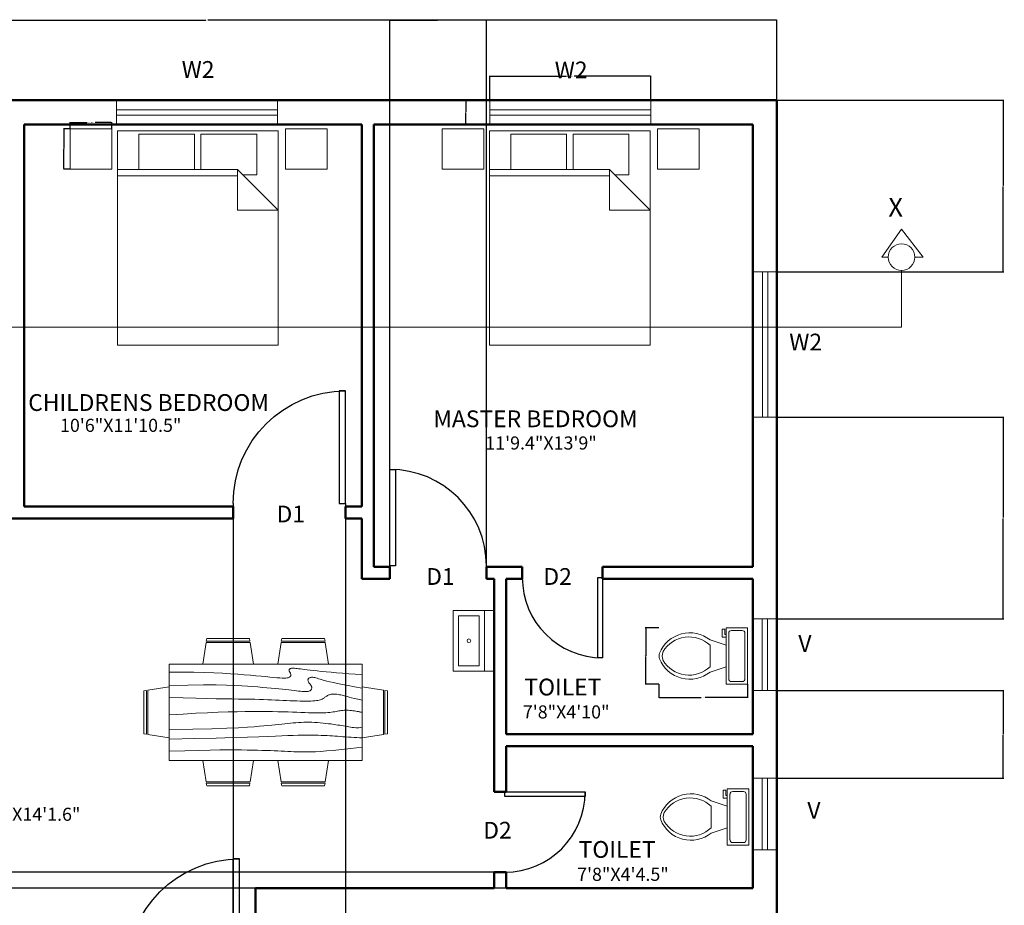
# Model space of a CAD drawing. Units: inches. Extents: x 7359 to 7979, y 33027 to 34263.
# Tile 32 of 32: x 7601 to 7969, y 33933 to 34263. Entities that reach past the tile are written whole.
import ezdxf

# ---------------------------------------------------------------- set-up
doc = ezdxf.new("R2010")
doc.units = ezdxf.units.IN
for name, color, linetype, lineweight in [('A-ANNO-DIMS', 2, 'Continuous', 18), ('A-ANNO-SYMB', 7, 'Continuous', 18), ('A-ANNO-TEXT', 3, 'Continuous', 18), ('A-AREA-IDEN', 7, 'Continuous', 18), ('A-DOOR', 3, 'Continuous', 25), ('A-FLOR-FIXT', 9, 'Continuous', 18), ('A-FURN', 8, 'Continuous', 18), ('A-GLAZ', 4, 'Continuous', 18), ('A-WALL', 7, 'Continuous', 50)]:
    doc.layers.add(name, color=color, linetype=linetype, lineweight=lineweight)
doc.styles.get("Standard").update_dxf_attribs({"font": 'arial.ttf'})
doc.dimstyles.get("Standard").update_dxf_attribs({"dimtxt": 0.18, "dimasz": 0.18, "dimexe": 0.18, "dimexo": 0.0625, "dimgap": 0.09, "dimtad": 0, "dimtih": 1, "dimtoh": 1, "dimdec": 4, "dimzin": 0, "dimdsep": 46, "dimtxsty": 'Standard', "dimcen": 0.09, "dimadec": 0, "dimazin": 0, "dimtfac": 1, "dimtdec": 4, "dimtofl": 0, "dimtmove": 0, "dimatfit": 3, "dimfxl": 1, "dimtolj": 1, "dimtzin": 0, "dimarcsym": 0})

# ---------------------------------------------------------------- blocks, each defined once
blk = doc.blocks.new('*U2')
for p, q in [((0, 0), (0, -100)), ((750, 0), (750, -100))]:
    blk.add_line(p, q)
blk.add_lwpolyline([(0, 0), (0, 750), (43.75, 750), (43.75, 0)], close=True)
blk.add_arc((0, 0), 750, 0, 90)
blk = doc.blocks.new('Dining Set - 36 x 72 in.')
for p, q in [((-22.2343, 26.00059), (-23.4847, 17.99762)), ((-22.2304, 26), (-5.7608, 26)), ((-22, 27.5), (-22.1562, 26.50042)), ((-5.8416, 26.5), (-22.1534, 26.5)), ((-22, 27.5), (-6, 27.5)), ((-5.8437, 26.49966), (-6, 27.5)), ((-4.5152, 17.99762), (-5.7655, 25.99926)), ((5.7657, 26.00059), (4.5153, 17.99762)), ((5.7696, 26), (22.2392, 26)), ((6, 27.5), (5.8438, 26.50042)), ((22.1584, 26.5), (5.8466, 26.5)), ((6, 27.5), (22, 27.5)), ((22.1563, 26.49966), (22, 27.5)), ((23.4848, 17.99762), (22.2345, 25.99926)), ((36, 18), (-36, 18)), ((-36, 18), (-36, -18)), ((36, -18), (36, 18)), ((-45.5, 8), (-44.5004, 8.15617)), ((-45.5, 8), (-45.5, -8)), ((-44.5, -8.15843), (-44.5, 8.15338)), ((-44.0006, 8.23428), (-35.9976, 9.48474)), ((-44, 8.23041), (-44, -8.23915)), ((44.0006, 8.23428), (35.9976, 9.48474)), ((44, 8.23041), (44, -8.23915)), ((44.5, -8.15843), (44.5, 8.15338)), ((45.5, 8), (44.5005, 8.15617)), ((45.5, 8), (45.5, -8)), ((-44.4997, -8.15631), (-45.5, -8)), ((-35.9976, -9.48476), (-43.9993, -8.2345)), ((35.9976, -9.48476), (43.9993, -8.2345)), ((44.4997, -8.15631), (45.5, -8)), ((-36, -18), (36, -18)), ((-22.2343, -26.0006), (-23.4847, -17.99762)), ((-4.5152, -17.99762), (-5.7655, -25.99928)), ((5.7657, -26.0006), (4.5153, -17.99762)), ((23.4848, -17.99762), (22.2345, -25.99928)), ((-22.2304, -26), (-5.7608, -26)), ((-22, -27.5), (-22.1562, -26.50044)), ((-5.8416, -26.5), (-22.1534, -26.5)), ((-22, -27.5), (-6, -27.5)), ((-5.8437, -26.49967), (-6, -27.5)), ((5.7696, -26), (22.2392, -26)), ((6, -27.5), (5.8438, -26.50044)), ((22.1584, -26.5), (5.8466, -26.5)), ((6, -27.5), (22, -27.5)), ((22.1563, -26.49967), (22, -27.5))]:
    blk.add_line(p, q)
for points in [[(-36, 15), (-31.1772, 14.97754), (-26.8079, 14.91406), (-22.8538, 14.81543), (-19.276, 14.6875), (-16.0362, 14.53613), (-13.0957, 14.36718), (-10.4159, 14.18652), (-7.9583, 14), (-5.6904, 13.81315), (-3.6035, 13.63021), (-1.6954, 13.45508), (0.0365, 13.29166), (1.5945, 13.14388), (2.9811, 13.01562), (4.1988, 12.9108), (5.25, 12.83333), (6.1393, 12.78613), (6.8802, 12.76823), (7.4883, 12.77767), (7.9792, 12.8125), (8.3685, 12.87077), (8.6719, 12.95052), (8.9049, 13.0498), (9.0833, 13.16666), (9.2205, 13.29899), (9.3216, 13.44401), (9.3895, 13.59879), (9.4271, 13.76041), (9.4373, 13.92594), (9.4232, 14.09245), (9.3875, 14.257), (9.3333, 14.41666), (9.2638, 14.56917), (9.1836, 14.71484), (9.0975, 14.85465), (9.0104, 14.98958), (8.9272, 15.1206), (8.8529, 15.2487), (8.7922, 15.37483), (8.75, 15.5), (8.7305, 15.62467), (8.7344, 15.74739), (8.7617, 15.86621), (8.8125, 15.97916), (8.8867, 16.08431), (8.9844, 16.17968), (9.1055, 16.26334), (9.25, 16.33333), (9.4189, 16.38802), (9.6172, 16.42708), (9.8506, 16.45052), (10.125, 16.45833), (10.4463, 16.45052), (10.8203, 16.42708), (11.2529, 16.38802), (11.75, 16.33333), (12.3184, 16.26318), (12.9694, 16.17838), (13.7151, 16.07991), (14.5677, 15.96875), (15.5395, 15.84586), (16.6426, 15.71224), (17.8893, 15.56884), (19.2917, 15.41666), (20.859, 15.25667), (22.5879, 15.08984), (24.4721, 14.91715), (26.5052, 14.73958), (28.6809, 14.5581), (30.9929, 14.3737), (33.4347, 14.18733), (36, 14)], [(-36, 10), (-28.9766, 10.14274), (-23.1725, 10.20442), (-18.4241, 10.19775), (-14.5677, 10.13541), (-11.4399, 10.03011), (-8.877, 9.89453), (-6.7154, 9.74137), (-4.7917, 9.58333), (-2.9698, 9.43082), (-1.2246, 9.28515), (0.4415, 9.14534), (2.026, 9.01041), (3.5266, 8.87939), (4.9408, 8.7513), (6.266, 8.62516), (7.5, 8.5), (8.6411, 8.37549), (9.6914, 8.2539), (10.6538, 8.13818), (11.5312, 8.03125), (12.3267, 7.93603), (13.043, 7.85547), (13.6831, 7.79248), (14.25, 7.75), (14.7471, 7.7303), (15.1797, 7.73307), (15.5537, 7.75732), (15.875, 7.80208), (16.1494, 7.86637), (16.3828, 7.94922), (16.5811, 8.04964), (16.75, 8.16666), (16.8944, 8.29915), (17.0143, 8.44531), (17.1089, 8.60319), (17.1771, 8.77083), (17.218, 8.94629), (17.2305, 9.1276), (17.2137, 9.31282), (17.1667, 9.5), (17.0895, 9.6875), (16.987, 9.875), (16.8649, 10.0625), (16.7292, 10.25), (16.5856, 10.4375), (16.4401, 10.625), (16.2985, 10.8125), (16.1667, 11), (16.05, 11.18733), (15.9518, 11.3737), (15.8752, 11.5581), (15.8229, 11.73958), (15.798, 11.91715), (15.8034, 12.08984), (15.842, 12.25667), (15.9167, 12.41666), (16.0295, 12.56836), (16.1784, 12.70833), (16.3605, 12.83268), (16.5729, 12.9375), (16.8127, 13.01888), (17.0768, 13.07291), (17.3625, 13.0957), (17.6667, 13.08333), (17.9894, 13.03312), (18.3418, 12.94726), (18.7382, 12.82918), (19.1927, 12.68229), (19.7195, 12.51001), (20.3327, 12.31575), (21.0465, 12.10294), (21.875, 11.875), (22.8357, 11.63354), (23.959, 11.37304), (25.2786, 11.08618), (26.8282, 10.76562), (28.6414, 10.40405), (30.752, 9.99414), (33.1936, 9.52856), (36, 9)], [(-36, 5.5), (-30.7157, 5.3348), (-26.069, 5.20963), (-21.9946, 5.11767), (-18.4271, 5.05208), (-15.3009, 5.00602), (-12.5508, 4.97265), (-10.1112, 4.94515), (-7.9167, 4.91666), (-5.909, 4.88167), (-4.0586, 4.83984), (-2.3429, 4.79215), (-0.7396, 4.73958), (0.7739, 4.6831), (2.22, 4.6237), (3.6213, 4.56233), (5, 4.5), (6.373, 4.43782), (7.7344, 4.3776), (9.0723, 4.32129), (10.375, 4.27083), (11.6309, 4.22819), (12.8281, 4.19531), (13.9551, 4.17415), (15, 4.16666), (15.954, 4.17448), (16.819, 4.19791), (17.6001, 4.23698), (18.3021, 4.29166), (18.9299, 4.36198), (19.4883, 4.44791), (19.9823, 4.54948), (20.4167, 4.66666), (20.7969, 4.79899), (21.1302, 4.94401), (21.4245, 5.09879), (21.6875, 5.26041), (21.9271, 5.42594), (22.1511, 5.59245), (22.3672, 5.757), (22.5834, 5.91666), (22.8065, 6.06868), (23.0404, 6.21093), (23.2879, 6.34147), (23.5521, 6.45833), (23.8358, 6.55957), (24.142, 6.64323), (24.4735, 6.70735), (24.8334, 6.75), (25.2235, 6.76969), (25.642, 6.76692), (26.0858, 6.74267), (26.5521, 6.69791), (27.0379, 6.63362), (27.5404, 6.55078), (28.0565, 6.45036), (28.5834, 6.33333), (29.1242, 6.19987), (29.7071, 6.04687), (30.3661, 5.87044), (31.1354, 5.66666), (32.0493, 5.43164), (33.142, 5.16146), (34.4475, 4.85221), (36, 4.5)], [(-36, -1), (-30.7915, -0.6591), (-26.0195, -0.38216), (-21.6519, -0.16284), (-17.6563, 0.00521), (-14.0005, 0.12833), (-10.6523, 0.21289), (-7.5796, 0.26522), (-4.75, 0.29166), (-2.134, 0.29793), (0.2878, 0.28711), (2.5317, 0.26163), (4.6146, 0.22396), (6.5529, 0.17651), (8.3633, 0.12174), (10.0623, 0.06209), (11.6667, 0), (13.1899, -0.06201), (14.6341, -0.1211), (15.9982, -0.17432), (17.2813, -0.21875), (18.4823, -0.25147), (19.6003, -0.26953), (20.6343, -0.27002), (21.5834, -0.25), (22.4481, -0.20768), (23.2357, -0.14584), (23.9549, -0.06836), (24.6146, 0.02083), (25.2235, 0.11784), (25.7904, 0.21875), (26.3241, 0.31966), (26.8334, 0.41666), (27.3265, 0.50618), (27.8099, 0.58593), (28.2894, 0.65397), (28.7709, 0.70833), (29.2601, 0.74707), (29.763, 0.76823), (30.2855, 0.76985), (30.8334, 0.75), (31.4088, 0.70784), (31.9994, 0.64713), (32.589, 0.57275), (33.1615, 0.48958), (33.7008, 0.4025), (34.1908, 0.3164), (34.6153, 0.23616), (34.9584, 0.16666), (35.2099, 0.11165), (35.3848, 0.07031), (35.504, 0.04069), (35.5886, 0.02083), (35.6594, 0.00879), (35.7377, 0.0026), (35.8442, 0.00032), (36, 0)], [(-36, -6.5), (-27.1843, -6.31267), (-20.084, -6.1263), (-14.469, -5.9419), (-10.1094, -5.76042), (-6.7752, -5.58285), (-4.2363, -5.41016), (-2.2629, -5.24333), (-0.625, -5.08334), (0.8708, -4.93099), (2.2715, -4.78646), (3.5872, -4.64974), (4.8281, -4.52084), (6.0046, -4.39974), (7.127, -4.28646), (8.2053, -4.18099), (9.25, -4.08334), (10.2705, -3.99382), (11.2734, -3.91407), (12.2647, -3.84603), (13.25, -3.79167), (14.2354, -3.75293), (15.2266, -3.73177), (16.2295, -3.73015), (17.25, -3.75), (18.2912, -3.79248), (19.3451, -3.85547), (20.4009, -3.93604), (21.4479, -4.03125), (22.4754, -4.13819), (23.4727, -4.25391), (24.4289, -4.37549), (25.3334, -4.5), (26.1785, -4.62492), (26.9694, -4.74935), (27.7145, -4.87281), (28.4219, -4.99479), (29.1, -5.11483), (29.7572, -5.23242), (30.4016, -5.34709), (31.0417, -5.45834), (31.6837, -5.56437), (32.3262, -5.65821), (32.9658, -5.73153), (33.599, -5.77604), (34.2224, -5.78345), (34.8327, -5.74545), (35.4264, -5.65373), (36, -5.5)], [(-36, -10), (-26.4022, -9.81299), (-18.4675, -9.62891), (-11.9839, -9.45069), (-6.7396, -9.28125), (-2.5226, -9.12354), (0.8789, -8.98047), (3.6769, -8.85498), (6.0833, -8.75), (8.2767, -8.66765), (10.3021, -8.60677), (12.1712, -8.56543), (13.8958, -8.54167), (15.4876, -8.53353), (16.9583, -8.53907), (18.3197, -8.55632), (19.5834, -8.58334), (20.7616, -8.61841), (21.8685, -8.66081), (22.9188, -8.71004), (23.9271, -8.76563), (24.9081, -8.82707), (25.8763, -8.89388), (26.8465, -8.96558), (27.8334, -9.04167), (28.8474, -9.12118), (29.8828, -9.20117), (30.93, -9.27824), (31.9792, -9.34896), (33.0205, -9.40991), (34.0443, -9.45768), (35.0407, -9.48885), (36, -9.5)], [(-36, -14.5), (-30.0881, -14.33513), (-25.0332, -14.21224), (-20.7312, -14.12647), (-17.0781, -14.07292), (-13.97, -14.04671), (-11.3027, -14.04297), (-8.9724, -14.05681), (-6.875, -14.08334), (-4.9224, -14.11833), (-3.0905, -14.16016), (-1.3709, -14.20785), (0.2448, -14.26042), (1.7647, -14.3169), (3.1973, -14.3763), (4.5507, -14.43767), (5.8333, -14.5), (7.0554, -14.5621), (8.235, -14.62175), (9.3922, -14.67652), (10.5469, -14.72396), (11.7192, -14.76164), (12.929, -14.78711), (14.1965, -14.79794), (15.5417, -14.79167), (16.9933, -14.76424), (18.6152, -14.70508), (20.4804, -14.60197), (22.6615, -14.44271), (25.2312, -14.21509), (28.2624, -13.9069), (31.8277, -13.50594), (36, -13)]]:
    blk.add_lwpolyline(points)
blk = doc.blocks.new('Bed - Queen')
for p, q in [((0, -80.00003), (0, 0)), ((0, 0), (59.99999, 0)), ((59.99999, 0), (59.99999, -80.00003)), ((7.99999, -1.2), (28.79998, -1.2)), ((7.99999, -14.4), (7.99999, -1.2)), ((28.79998, -1.2), (28.79998, -14.4)), ((31.19999, -1.2), (51.99999, -1.2)), ((31.19999, -14.4), (31.19999, -1.2)), ((51.99999, -1.2), (51.99999, -16.4)), ((0, -14.4), (44.8, -14.4)), ((59.99999, -29.6), (44.8, -14.4)), ((44.8, -14.4), (44.8, -29.6)), ((44.8, -16.8), (0, -16.8)), ((51.99999, -16.4), (46.79936, -16.4)), ((44.8, -29.6), (59.99999, -29.6)), ((59.99999, -80.00003), (0, -80.00003))]:
    blk.add_line(p, q)
blk = doc.blocks.new('Toilet - top')
for p, q in [((9.5, -6), (9.5, -2)), ((-10, -8.5), (-8, -8.5)), ((-10, -9.5), (-10, -8.5)), ((-7, -9.5), (-10, -9.5)), ((-8, -8.5), (-8, -8)), ((-7, -8), (-7, -9.5)), ((-4, -8), (-6, -14)), ((4, -8), (6, -14)), ((4, -14), (-4, -14))]:
    blk.add_line(p, q)
blk.add_lwpolyline([(10.5, -8), (10.5, 0), (-10.5, 0), (-10.5, -8)], close=True)
for points in [[(-9.5, -2), (-9.5, -6)], [(8.5, -1), (-8.5, -1)], [(-8.5, -7), (8.5, -7)]]:
    blk.add_lwpolyline(points)
for centre, radius, start, end in [((-8.62, -1.88), 0.884, 81.8699, 188.1301), ((8.62, -1.88), 0.884, 351.8699, 98.1301), ((-8.62, -6.12), 0.884, 171.8699, 278.1301), ((8.62, -6.12), 0.884, 261.8699, 8.1301), ((3.52, -21.58), 12.17, 141.4691, 247.9714), ((4.2, -21.82), 11.33, 136.3677, 238.9468), ((-3.52, -21.58), 12.17, 292.0284, 38.5307), ((-4.2, -21.82), 11.33, 301.053, 43.6321), ((0, -27.88), 4, 245.7318, 294.2682), ((0, -29), 4, 254.8605, 285.1395)]:
    blk.add_arc(centre, radius, start, end)
blk = doc.blocks.new('TABLE-BEDSIDE')
blk.add_lwpolyline([(0, 15), (15.54, 15), (15.54, 0), (0, 0)], close=True)
blk = doc.blocks.new('BASIN-WALL')
for points in [[(11.75, 22.71), (0, 22.71), (0, 0), (11.75, 0)], [(15.29, 22.71), (11.75, 22.71), (11.75, 0), (15.29, 0)], [(9.75, 20.71), (2, 20.71), (2, 2), (9.75, 2)]]:
    blk.add_lwpolyline(points, close=True)
blk.add_circle((5.88, 11.36), 0.663)
blk = doc.blocks.new('SECTION-HEAD')
for p, q in [((0, 4.98), (7.32, 15.43)), ((7.32, 15.43), (15.39, 4.98)), ((2.34, 4.98), (0, 4.98)), ((12.3, 4.98), (15.39, 4.98))]:
    blk.add_line(p, q)
blk.add_circle((7.32, 4.98), 4.98)
blk = doc.blocks.new('WINDOW-W2-BEDROOM')
for p, q in [((0, 0), (0, 9)), ((60.05, 0), (60.05, 9)), ((60.05, 5.5), (0, 5.5)), ((60.05, 3.5), (0, 3.5))]:
    blk.add_line(p, q)
blk = doc.blocks.new('WINDOW-W2-SIDE')
for p, q in [((0, 54.21), (9, 54.21)), ((3.61, 0), (3.61, 54.21)), ((5.61, 0), (5.61, 54.21)), ((0.22, 0), (9, 0))]:
    blk.add_line(p, q)
blk = doc.blocks.new('VENT-V')
for p, q in [((0, 26.78), (9, 26.78)), ((3.5, 0), (3.5, 26.78)), ((5.5, 0), (5.5, 26.78)), ((0, 0), (9, 0))]:
    blk.add_line(p, q)
blk = doc.blocks.new('*D24')
at = {"layer": 'A-ANNO-DIMS', "color": 0, "lineweight": -2, "transparency": 16777216}
for p, q in [((7620.26, 34222.75), (7620.26, 34225.2)), ((7620.44, 34225.02), (7626.49, 34225.02)), ((7635.62, 34225.02), (7629.57, 34225.02)), ((7635.8, 34222.75), (7635.8, 34225.2))]:
    blk.add_line(p, q, dxfattribs=at)
at = {"layer": 'A-ANNO-DIMS', "color": 0, "transparency": 16777216}
for points in [[(7620.44, 34225.05), (7620.44, 34224.99), (7620.26, 34225.02)], [(7635.62, 34225.05), (7635.62, 34224.99), (7635.8, 34225.02)]]:
    blk.add_solid(points, dxfattribs=at)
at = {"layer": 'Defpoints', "color": 0, "transparency": 16777216}
for p in [(7620.26, 34222.69), (7635.8, 34225.02), (7635.8, 34222.69)]:
    blk.add_point(p, dxfattribs=at)
at = {"layer": 'A-ANNO-DIMS', "color": 0, "transparency": 16777216, "insert": (7628.03, 34225.02), "char_height": 0.18, "attachment_point": 5}
blk.add_mtext('\\A1;BEDSIDE TABLE 16 TYP.', dxfattribs=at)
blk = doc.blocks.new('*D25')
at = {"layer": 'A-ANNO-DIMS', "color": 0, "lineweight": -2, "transparency": 16777216}
for p, q in [((7620.2, 34222.69), (7617.75, 34222.69)), ((7617.93, 34222.51), (7617.93, 34215.37)), ((7617.93, 34207.87), (7617.93, 34215.01)), ((7620.2, 34207.69), (7617.75, 34207.69))]:
    blk.add_line(p, q, dxfattribs=at)
at = {"layer": 'A-ANNO-DIMS', "color": 0, "transparency": 16777216}
for points in [[(7617.9, 34222.51), (7617.96, 34222.51), (7617.93, 34222.69)], [(7617.9, 34207.87), (7617.96, 34207.87), (7617.93, 34207.69)]]:
    blk.add_solid(points, dxfattribs=at)
at = {"layer": 'Defpoints', "color": 0, "transparency": 16777216}
for p in [(7617.93, 34222.69), (7620.26, 34222.69), (7620.26, 34207.69)]:
    blk.add_point(p, dxfattribs=at)
at = {"layer": 'A-ANNO-DIMS', "color": 0, "transparency": 16777216, "insert": (7617.93, 34215.19), "char_height": 0.18, "attachment_point": 5}
blk.add_mtext('\\A1;15 TYP.', dxfattribs=at)
blk = doc.blocks.new('*D30')
at = {"layer": 'A-ANNO-DIMS', "color": 0, "lineweight": -2, "transparency": 16777216}
for p, q in [((7840.01, 34015.44), (7840.01, 34010.37)), ((7873.06, 34015.44), (7873.06, 34010.37)), ((7840.19, 34010.55), (7855.76, 34010.55)), ((7872.88, 34010.55), (7857.31, 34010.55))]:
    blk.add_line(p, q, dxfattribs=at)
at = {"layer": 'A-ANNO-DIMS', "color": 0, "transparency": 16777216}
for points in [[(7840.19, 34010.58), (7840.19, 34010.52), (7840.01, 34010.55)], [(7872.88, 34010.58), (7872.88, 34010.52), (7873.06, 34010.55)]]:
    blk.add_solid(points, dxfattribs=at)
at = {"layer": 'Defpoints', "color": 0, "transparency": 16777216}
for p in [(7840.01, 34015.5), (7873.06, 34015.5), (7873.06, 34010.55)]:
    blk.add_point(p, dxfattribs=at)
at = {"layer": 'A-ANNO-DIMS', "color": 0, "transparency": 16777216, "insert": (7856.54, 34010.55), "char_height": 0.18, "attachment_point": 5}
blk.add_mtext('\\A1;WC 33 TYP.', dxfattribs=at)
blk = doc.blocks.new('*D31')
at = {"layer": 'A-ANNO-DIMS', "color": 0, "lineweight": -2, "transparency": 16777216}
for p, q in [((7839.95, 34036.5), (7834.88, 34036.5)), ((7835.06, 34036.32), (7835.06, 34026.18)), ((7835.06, 34015.68), (7835.06, 34025.82)), ((7839.95, 34015.5), (7834.88, 34015.5))]:
    blk.add_line(p, q, dxfattribs=at)
at = {"layer": 'A-ANNO-DIMS', "color": 0, "transparency": 16777216}
for points in [[(7835.03, 34036.32), (7835.09, 34036.32), (7835.06, 34036.5)], [(7835.03, 34015.68), (7835.09, 34015.68), (7835.06, 34015.5)]]:
    blk.add_solid(points, dxfattribs=at)
at = {"layer": 'Defpoints', "color": 0, "transparency": 16777216}
for p in [(7840.01, 34036.5), (7835.06, 34015.5), (7840.01, 34015.5)]:
    blk.add_point(p, dxfattribs=at)
at = {"layer": 'A-ANNO-DIMS', "color": 0, "transparency": 16777216, "insert": (7835.06, 34026), "char_height": 0.18, "attachment_point": 5}
blk.add_mtext('\\A1;21 TYP.', dxfattribs=at)
blk = doc.blocks.new('*D32')
at = {"layer": 'A-ANNO-DIMS', "color": 0, "lineweight": -2, "transparency": 16777216}
for p, q in [((7776.9, 34233.4), (7776.9, 34242.52)), ((7777.08, 34242.34), (7805.49, 34242.34)), ((7836.77, 34242.34), (7808.36, 34242.34)), ((7836.95, 34233.4), (7836.95, 34242.52))]:
    blk.add_line(p, q, dxfattribs=at)
at = {"layer": 'A-ANNO-DIMS', "color": 0, "transparency": 16777216}
for points in [[(7777.08, 34242.37), (7777.08, 34242.31), (7776.9, 34242.34)], [(7836.77, 34242.37), (7836.77, 34242.31), (7836.95, 34242.34)]]:
    blk.add_solid(points, dxfattribs=at)
at = {"layer": 'Defpoints', "color": 0, "transparency": 16777216}
for p in [(7836.95, 34242.34), (7776.9, 34233.33), (7836.95, 34233.33)]:
    blk.add_point(p, dxfattribs=at)
at = {"layer": 'A-ANNO-DIMS', "color": 0, "transparency": 16777216, "insert": (7806.92, 34242.34), "char_height": 0.18, "attachment_point": 5}
blk.add_mtext('\\A1;BEDROOM W2 60 TYP.', dxfattribs=at)
blk = doc.blocks.new('*D33')
at = {"layer": 'A-ANNO-DIMS', "color": 0, "lineweight": -2, "transparency": 16777216}
for p, q in [((7776.84, 34233.33), (7767.71, 34233.33)), ((7767.89, 34233.15), (7767.89, 34229.02)), ((7767.89, 34224.51), (7767.89, 34228.65)), ((7776.84, 34224.33), (7767.71, 34224.33))]:
    blk.add_line(p, q, dxfattribs=at)
at = {"layer": 'A-ANNO-DIMS', "color": 0, "transparency": 16777216}
for points in [[(7767.86, 34233.15), (7767.92, 34233.15), (7767.89, 34233.33)], [(7767.86, 34224.51), (7767.92, 34224.51), (7767.89, 34224.33)]]:
    blk.add_solid(points, dxfattribs=at)
at = {"layer": 'Defpoints', "color": 0, "transparency": 16777216}
for p in [(7767.89, 34233.33), (7776.9, 34233.33), (7776.9, 34224.33)]:
    blk.add_point(p, dxfattribs=at)
at = {"layer": 'A-ANNO-DIMS', "color": 0, "transparency": 16777216, "insert": (7767.89, 34228.83), "char_height": 0.18, "attachment_point": 5}
blk.add_mtext('\\A1;9 TYP.', dxfattribs=at)
blk = doc.blocks.new('*D64')
at = {"layer": 'A-ANNO-DIMS', "color": 0, "lineweight": -2, "transparency": 16777216}
for p, q in [((7458.59, 34233.4), (7458.59, 34263.41)), ((7458.77, 34263.23), (7670.89, 34263.23)), ((7883.81, 34263.23), (7671.69, 34263.23)), ((7883.99, 34233.4), (7883.99, 34263.41))]:
    blk.add_line(p, q, dxfattribs=at)
at = {"layer": 'A-ANNO-DIMS', "color": 0, "transparency": 16777216}
for points in [[(7458.77, 34263.26), (7458.77, 34263.2), (7458.59, 34263.23)], [(7883.81, 34263.26), (7883.81, 34263.2), (7883.99, 34263.23)]]:
    blk.add_solid(points, dxfattribs=at)
at = {"layer": 'Defpoints', "color": 0, "transparency": 16777216}
for p in [(7883.99, 34263.23), (7458.59, 34233.33), (7883.99, 34233.33)]:
    blk.add_point(p, dxfattribs=at)
at = {"layer": 'A-ANNO-DIMS', "color": 0, "transparency": 16777216, "insert": (7671.29, 34263.23), "char_height": 0.18, "attachment_point": 5}
blk.add_mtext('\\A1;425.4', dxfattribs=at)
blk = doc.blocks.new('*D69')
at = {"layer": 'A-ANNO-DIMS', "color": 0, "lineweight": -2, "transparency": 16777216}
for p, q in [((7681.09, 34081.77), (7681.09, 33632.31)), ((7723.09, 34081.77), (7723.09, 33632.31)), ((7681.27, 33632.49), (7701.87, 33632.49)), ((7722.91, 33632.49), (7702.31, 33632.49))]:
    blk.add_line(p, q, dxfattribs=at)
at = {"layer": 'A-ANNO-DIMS', "color": 0, "transparency": 16777216}
for points in [[(7681.27, 33632.52), (7681.27, 33632.46), (7681.09, 33632.49)], [(7722.91, 33632.52), (7722.91, 33632.46), (7723.09, 33632.49)]]:
    blk.add_solid(points, dxfattribs=at)
at = {"layer": 'Defpoints', "color": 0, "transparency": 16777216}
for p in [(7681.09, 34081.83), (7723.09, 34081.83), (7723.09, 33632.49)]:
    blk.add_point(p, dxfattribs=at)
at = {"layer": 'A-ANNO-DIMS', "color": 0, "transparency": 16777216, "insert": (7702.09, 33632.49), "char_height": 0.18, "attachment_point": 5}
blk.add_mtext('\\A1;42', dxfattribs=at)
blk = doc.blocks.new('*D70')
at = {"layer": 'A-ANNO-DIMS', "color": 0, "lineweight": -2, "transparency": 16777216}
for p, q in [((7739.59, 34059.4), (7739.59, 34263.41)), ((7739.77, 34263.23), (7757.37, 34263.23)), ((7775.41, 34263.23), (7757.81, 34263.23)), ((7775.59, 34059.4), (7775.59, 34263.41))]:
    blk.add_line(p, q, dxfattribs=at)
at = {"layer": 'A-ANNO-DIMS', "color": 0, "transparency": 16777216}
for points in [[(7739.77, 34263.26), (7739.77, 34263.2), (7739.59, 34263.23)], [(7775.41, 34263.26), (7775.41, 34263.2), (7775.59, 34263.23)]]:
    blk.add_solid(points, dxfattribs=at)
at = {"layer": 'Defpoints', "color": 0, "transparency": 16777216}
for p in [(7775.59, 34263.23), (7739.59, 34059.33), (7775.59, 34059.33)]:
    blk.add_point(p, dxfattribs=at)
at = {"layer": 'A-ANNO-DIMS', "color": 0, "transparency": 16777216, "insert": (7757.59, 34263.23), "char_height": 0.18, "attachment_point": 5}
blk.add_mtext('\\A1;36', dxfattribs=at)
blk = doc.blocks.new('*D75')
at = {"layer": 'A-ANNO-DIMS', "color": 0, "lineweight": -2, "transparency": 16777216}
for p, q in [((7884.05, 34233.33), (7968.68, 34233.33)), ((7968.5, 34233.15), (7968.5, 34201.53)), ((7968.5, 34169.55), (7968.5, 34201.17)), ((7884.05, 34169.37), (7968.68, 34169.37))]:
    blk.add_line(p, q, dxfattribs=at)
at = {"layer": 'A-ANNO-DIMS', "color": 0, "transparency": 16777216}
for points in [[(7968.47, 34233.15), (7968.53, 34233.15), (7968.5, 34233.33)], [(7968.47, 34169.55), (7968.53, 34169.55), (7968.5, 34169.37)]]:
    blk.add_solid(points, dxfattribs=at)
at = {"layer": 'Defpoints', "color": 0, "transparency": 16777216}
for p in [(7883.99, 34233.33), (7883.99, 34169.37), (7968.5, 34169.37)]:
    blk.add_point(p, dxfattribs=at)
at = {"layer": 'A-ANNO-DIMS', "color": 0, "transparency": 16777216, "insert": (7968.5, 34201.35), "char_height": 0.18, "attachment_point": 5}
blk.add_mtext('\\A1;63.97', dxfattribs=at)
blk = doc.blocks.new('*D76')
at = {"layer": 'A-ANNO-DIMS', "color": 0, "lineweight": -2, "transparency": 16777216}
for p, q in [((7884.05, 34115.16), (7968.68, 34115.16)), ((7968.5, 34114.98), (7968.5, 34077.72)), ((7968.5, 34040.09), (7968.5, 34077.35)), ((7884.05, 34039.91), (7968.68, 34039.91))]:
    blk.add_line(p, q, dxfattribs=at)
at = {"layer": 'A-ANNO-DIMS', "color": 0, "transparency": 16777216}
for points in [[(7968.47, 34114.98), (7968.53, 34114.98), (7968.5, 34115.16)], [(7968.47, 34040.09), (7968.53, 34040.09), (7968.5, 34039.91)]]:
    blk.add_solid(points, dxfattribs=at)
at = {"layer": 'Defpoints', "color": 0, "transparency": 16777216}
for p in [(7883.99, 34115.16), (7883.99, 34039.91), (7968.5, 34039.91)]:
    blk.add_point(p, dxfattribs=at)
at = {"layer": 'A-ANNO-DIMS', "color": 0, "transparency": 16777216, "insert": (7968.5, 34077.53), "char_height": 0.18, "attachment_point": 5}
blk.add_mtext('\\A1;75.24', dxfattribs=at)
blk = doc.blocks.new('*D77')
at = {"layer": 'A-ANNO-DIMS', "color": 0, "lineweight": -2, "transparency": 16777216}
for p, q in [((7884.05, 34013.13), (7968.68, 34013.13)), ((7968.5, 34012.95), (7968.5, 33996.96)), ((7968.5, 33980.61), (7968.5, 33996.6)), ((7884.05, 33980.43), (7968.68, 33980.43))]:
    blk.add_line(p, q, dxfattribs=at)
at = {"layer": 'A-ANNO-DIMS', "color": 0, "transparency": 16777216}
for points in [[(7968.47, 34012.95), (7968.53, 34012.95), (7968.5, 34013.13)], [(7968.47, 33980.61), (7968.53, 33980.61), (7968.5, 33980.43)]]:
    blk.add_solid(points, dxfattribs=at)
at = {"layer": 'Defpoints', "color": 0, "transparency": 16777216}
for p in [(7883.99, 34013.13), (7883.99, 33980.43), (7968.5, 33980.43)]:
    blk.add_point(p, dxfattribs=at)
at = {"layer": 'A-ANNO-DIMS', "color": 0, "transparency": 16777216, "insert": (7968.5, 33996.78), "char_height": 0.18, "attachment_point": 5}
blk.add_mtext('\\A1;32.705', dxfattribs=at)
blk = doc.blocks.new('*D84')
at = {"layer": 'A-ANNO-DIMS', "color": 0, "lineweight": -2, "transparency": 16777216}
for p, q in [((7782.93, 33945.33), (7359.41, 33945.33)), ((7359.59, 33945.15), (7359.59, 33942.52)), ((7782.93, 33939.33), (7359.41, 33939.33)), ((7359.59, 33939.51), (7359.59, 33942.15))]:
    blk.add_line(p, q, dxfattribs=at)
at = {"layer": 'A-ANNO-DIMS', "color": 0, "transparency": 16777216}
for points in [[(7359.56, 33945.15), (7359.62, 33945.15), (7359.59, 33945.33)], [(7359.56, 33939.51), (7359.62, 33939.51), (7359.59, 33939.33)]]:
    blk.add_solid(points, dxfattribs=at)
at = {"layer": 'Defpoints', "color": 0, "transparency": 16777216}
for p in [(7782.99, 33945.33), (7359.59, 33939.33), (7782.99, 33939.33)]:
    blk.add_point(p, dxfattribs=at)
at = {"layer": 'A-ANNO-DIMS', "color": 0, "transparency": 16777216, "insert": (7359.59, 33942.33), "char_height": 0.18, "attachment_point": 5}
blk.add_mtext('\\A1;6', dxfattribs=at)

msp = doc.modelspace()

# ---------------------------------------------------------------- linework, layer by layer
at = {"layer": 'A-ANNO-SYMB'}
for p, q in [((7930.5345, 34148.6536), (7930.5345, 34169.8623)), ((7396.8072, 34148.6536), (7930.5345, 34148.6536))]:
    msp.add_line(p, q, dxfattribs=at)
at = {"layer": 'A-WALL'}
for p, q in [((7458.5915, 34233.3339), (7883.9915, 34233.3339)), ((7883.9915, 34233.3339), (7883.9915, 33764.8339)), ((7603.0915, 34224.3339), (7603.0915, 34081.8339)), ((7603.0915, 34224.3339), (7729.0915, 34224.3339)), ((7729.0915, 34224.3339), (7729.0915, 34081.8339)), ((7733.5915, 34224.3339), (7733.5915, 34059.3339)), ((7733.5915, 34224.3339), (7874.9915, 34224.3339)), ((7874.9915, 34224.3339), (7874.9915, 34059.3339)), ((7729.0915, 34094.8339), (7729.0915, 34081.8339)), ((7603.0915, 34081.8339), (7681.0915, 34081.8339)), ((7681.0915, 34081.8339), (7681.0915, 34077.3339)), ((7723.0915, 34081.8339), (7723.0915, 34077.3339)), ((7723.0915, 34081.8339), (7729.0915, 34081.8339)), ((7592.5915, 34077.3339), (7681.0915, 34077.3339)), ((7723.0915, 34077.3339), (7729.0915, 34077.3339)), ((7729.0915, 34077.3339), (7729.0915, 34054.8339)), ((7733.5915, 34059.3339), (7739.5915, 34059.3339)), ((7739.5915, 34059.3339), (7739.5915, 34054.8339)), ((7775.5915, 34059.3339), (7775.5915, 34054.8339)), ((7775.5915, 34059.3339), (7788.9915, 34059.3339)), ((7788.9915, 34054.8339), (7788.9915, 34059.3339)), ((7818.9915, 34054.8339), (7818.9915, 34059.3339)), ((7818.9915, 34059.3339), (7874.9915, 34059.3339)), ((7729.0915, 34054.8339), (7739.5915, 34054.8339)), ((7775.5915, 34054.8339), (7778.4915, 34054.8339)), ((7778.4915, 34054.8339), (7778.4915, 33975.3339)), ((7782.9915, 34054.8339), (7782.9915, 33996.8339)), ((7782.9915, 34054.8339), (7788.9915, 34054.8339)), ((7818.9915, 34054.8339), (7874.9915, 34054.8339)), ((7874.9915, 34054.8339), (7874.9915, 33996.8339)), ((7782.9915, 33996.8339), (7874.9915, 33996.8339)), ((7782.9915, 33992.3339), (7874.9915, 33992.3339)), ((7782.9915, 33992.3339), (7782.9915, 33975.3339)), ((7874.9915, 33992.3339), (7874.9915, 33939.3339)), ((7778.4915, 33975.3339), (7782.9915, 33975.3339)), ((7778.4915, 33945.3339), (7782.9915, 33945.3339)), ((7778.4915, 33945.3339), (7778.4915, 33939.3339)), ((7782.9915, 33945.3339), (7782.9915, 33939.3339)), ((7689.4915, 33939.3339), (7778.4915, 33939.3339)), ((7689.4915, 33939.3339), (7689.4915, 33907.2339)), ((7782.9915, 33939.3339), (7874.9915, 33939.3339))]:
    msp.add_line(p, q, dxfattribs=at)

# ---------------------------------------------------------------- block references
at = {"layer": 'A-ANNO-SYMB'}
msp.add_blockref('SECTION-HEAD', (7923.2143, 34169.862), dxfattribs=at)
at = {"layer": 'A-DOOR'}
for p, xscale, yscale, zscale in [((7723.0915, 34082.9339), -0.0559999819687567, 0.0559999819687567, 0.0559999819687567), ((7739.5915, 34059.6339), 0.0479999999999996, 0.0479999999999996, 0.0479999999999996), ((7683.4915, 33908.3339), -0.0559999819687567, 0.0559999819687567, 0.0559999819687567)]:
    msp.add_blockref('*U2', p, dxfattribs=dict(at, xscale=xscale, yscale=yscale, zscale=zscale))
at = {"layer": 'A-DOOR', "xscale": 0.0399999999999999, "yscale": 0.0399999999999999, "zscale": 0.0399999999999999}
for p, rotation in [((7818.9915, 34055.3339), 180), ((7782.4915, 33975.3339), 270)]:
    msp.add_blockref('*U2', p, dxfattribs=dict(at, rotation=rotation))
at = {"layer": 'A-FLOR-FIXT'}
msp.add_blockref('BASIN-WALL', (7763.198, 34020.335), dxfattribs=at)
at = {"layer": 'A-FLOR-FIXT', "rotation": 270}
for p in [(7873.0612, 34026.0021), (7873.5108, 33965.9256)]:
    msp.add_blockref('Toilet - top', p, dxfattribs=at)
at = {"layer": 'A-FURN'}
for name, p in [('TABLE-BEDSIDE', (7620.261, 34207.688)), ('Bed - Queen', (7637.9007, 34221.9339)), ('TABLE-BEDSIDE', (7700.6011, 34207.688)), ('TABLE-BEDSIDE', (7759.1007, 34207.688)), ('Bed - Queen', (7776.7404, 34221.9339)), ('TABLE-BEDSIDE', (7839.4409, 34207.688)), ('Dining Set - 36 x 72 in.', (7693.2279, 34005.0152))]:
    msp.add_blockref(name, p, dxfattribs=at)
at = {"layer": 'A-GLAZ'}
for name, p in [('WINDOW-W2-BEDROOM', (7637.571, 34224.334)), ('WINDOW-W2-BEDROOM', (7776.899, 34224.334)), ('WINDOW-W2-SIDE', (7874.991, 34115.156)), ('VENT-V', (7874.991, 34013.133)), ('VENT-V', (7874.991, 33953.649))]:
    msp.add_blockref(name, p, dxfattribs=at)

# ---------------------------------------------------------------- texts
at = {"layer": 'A-ANNO-SYMB'}
msp.add_text('X', height=6.9459, dxfattribs=at).set_placement((7925.6142, 34189.9559))
at = {"layer": 'A-ANNO-TEXT'}
for s, height, p in [('W2', 6.25941, (7661.9079, 34241.7079)), ('W2', 6.25941, (7801.1223, 34241.5211)), ('W2', 6.25941, (7888.6338, 34140.0052)), ('D1', 6.25941, (7697.3021, 34075.8565)), ('D1', 6.25941, (7753.1493, 34052.5401)), ('D2', 6.25941, (7796.8821, 34052.5401)), ('V', 6.2594, (7892.0148, 34027.5431)), ('V', 6.2594, (7895.3708, 33965.2689)), ('D2', 6.25941, (7774.4294, 33957.8777))]:
    msp.add_text(s, height=height, dxfattribs=at).set_placement(p)
at = {"layer": 'A-AREA-IDEN'}
for s, height, p in [('CHILDRENS BEDROOM', 6.259411, (7604.6305, 34117.4435)), ('MASTER BEDROOM', 6.259411, (7755.8118, 34111.3774)), ('10\'6"X11\'10.5"', 4.885549, (7616.5063, 34109.6257)), ('11\'9.4"X13\'9"', 4.885549, (7775.2095, 34103.0431)), ('TOILET', 6.25941, (7789.7808, 34011.2958)), ('7\'8"X4\'10"', 4.88555, (7789.2175, 34002.7014)), ('25\'10.9"X14\'1.6"', 4.885549, (7573.2739, 33964.5127)), ('TOILET', 6.25941, (7810.0319, 33950.709)), ('7\'8"X4\'4.5"', 4.885549, (7809.4687, 33942.1146))]:
    msp.add_text(s, height=height, dxfattribs=at).set_placement(p)

# ---------------------------------------------------------------- dimensions: what is measured, and where the dimension line sits
at = {"layer": 'A-ANNO-DIMS'}
for base, p1, p2, override, picture, middle in [((7883.9915, 34263.2339), (7458.5915, 34233.3339), (7883.9915, 34233.3339), {"dimdec": 1, "dimlfac": 1, "dimrnd": 0, "dimzin": 0, "dimdsep": 46, "dimlunit": 2}, '*D64', (7671.2915, 34263.2339)), ((7775.5915, 34263.2339), (7739.5915, 34059.3339), (7775.5915, 34059.3339), {"dimdec": 0, "dimlfac": 1, "dimrnd": 0, "dimzin": 0, "dimdsep": 46, "dimlunit": 2}, '*D70', (7757.5915, 34263.2339)), ((7723.0915, 33632.4891), (7681.0915, 34081.8339), (7723.0915, 34081.8339), {"dimdec": 0, "dimlfac": 1, "dimrnd": 0, "dimzin": 0, "dimdsep": 46, "dimlunit": 2}, '*D69', (7702.0915, 33632.4891))]:
    dim = msp.add_linear_dim(base=base, p1=p1, p2=p2, dimstyle='Standard', override=override, dxfattribs=at)
    dim.commit()
    dim.dimension.update_dxf_attribs({"geometry": picture, "text_midpoint": middle})
for base, p1, p2, text, picture, middle in [((7836.9465, 34242.341), (7776.8991, 34233.3339), (7836.9465, 34233.3339), 'BEDROOM W2 <> TYP.', '*D32', (7806.9228, 34242.341)), ((7635.7994, 34225.0204), (7620.2614, 34222.6897), (7635.7994, 34222.6897), 'BEDSIDE TABLE <> TYP.', '*D24', (7628.0304, 34225.0204)), ((7873.0612, 34010.5452), (7840.015, 34015.5021), (7873.0612, 34015.5021), 'WC <> TYP.', '*D30', (7856.5381, 34010.5452))]:
    dim = msp.add_linear_dim(base=base, p1=p1, p2=p2, text=text, dimstyle='Standard', override={"dimdec": 0, "dimlfac": 1, "dimrnd": 0, "dimzin": 0, "dimdsep": 46, "dimlunit": 2}, dxfattribs=at)
    dim.commit()
    dim.dimension.update_dxf_attribs({"geometry": picture, "text_midpoint": middle})
for base, p1, p2, angle, picture, middle in [((7767.892, 34233.3339), (7776.8991, 34224.3339), (7776.8991, 34233.3339), 90, '*D33', (7767.892, 34228.8339)), ((7617.9307, 34222.6897), (7620.2614, 34207.6877), (7620.2614, 34222.6897), 90, '*D25', (7617.9307, 34215.1887)), ((7835.058, 34015.5021), (7840.015, 34036.5021), (7840.015, 34015.5021), 270, '*D31', (7835.058, 34026.0021))]:
    dim = msp.add_linear_dim(base=base, p1=p1, p2=p2, angle=angle, text='<> TYP.', dimstyle='Standard', override={"dimdec": 0, "dimlfac": 1, "dimrnd": 0, "dimzin": 0, "dimdsep": 46, "dimlunit": 2}, dxfattribs=at)
    dim.commit()
    dim.dimension.update_dxf_attribs({"geometry": picture, "text_midpoint": middle})
for base, p1, p2, override, picture, middle in [((7968.502, 34169.3688), (7883.9915, 34233.3339), (7883.9915, 34169.3688), {"dimdec": 2, "dimlfac": 1, "dimrnd": 0, "dimzin": 0, "dimdsep": 46, "dimlunit": 2}, '*D75', (7968.502, 34201.3514)), ((7968.502, 34039.912), (7883.9915, 34115.1562), (7883.9915, 34039.912), {"dimdec": 2, "dimlfac": 1, "dimrnd": 0, "dimzin": 0, "dimdsep": 46, "dimlunit": 2}, '*D76', (7968.502, 34077.5341)), ((7968.502, 33980.428), (7883.9915, 34013.1332), (7883.9915, 33980.428), {"dimdec": 3, "dimlfac": 1, "dimrnd": 0, "dimzin": 0, "dimdsep": 46, "dimlunit": 2}, '*D77', (7968.502, 33996.7806)), ((7359.5866, 33939.3339), (7782.9915, 33945.3339), (7782.9915, 33939.3339), {"dimdec": 0, "dimlfac": 1, "dimrnd": 0, "dimzin": 0, "dimdsep": 46, "dimlunit": 2}, '*D84', (7359.5866, 33942.3339))]:
    dim = msp.add_linear_dim(base=base, p1=p1, p2=p2, angle=90, dimstyle='Standard', override=override, dxfattribs=at)
    dim.commit()
    dim.dimension.update_dxf_attribs({"geometry": picture, "text_midpoint": middle})

doc.saveas('drawing.dxf')
